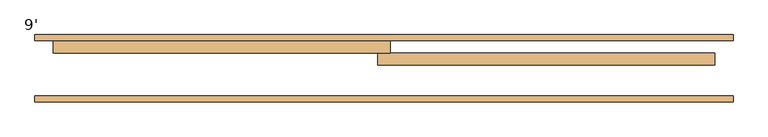
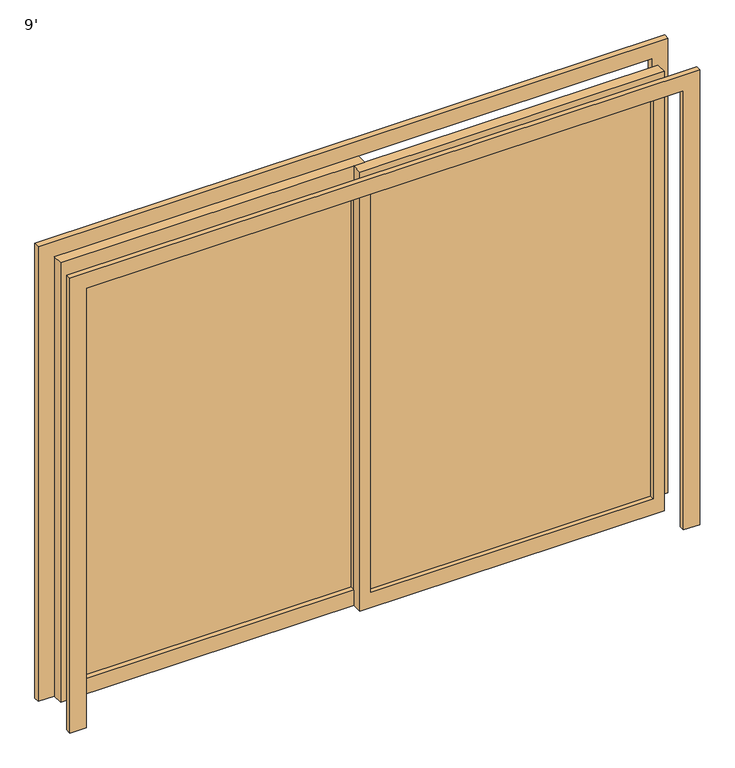
"""IFC4 building model written with IfcOpenShell, lengths in millimetres: door geometry, 9'."""

from ifc_helpers import new_model, si_unit, frame, origin, place, context, project, spatial, polyline, outline, extrude, source, transform, mapped, element, save


def door_9_db2a89ef(model_context):
    return source(origin(), model_context, "Body", "SweptSolid", [
        extrude(outline(polyline([(0.0, 1446.6), (2209.0, 1446.6), (2209.0, -1446.6), (0.0, -1446.6), (0.0, -1371.6), (2134.0, -1371.6), (2134.0, 1371.6), (0.0, 1371.6), (0.0, 1446.6)])), frame((0.0, 241.3, 0.0), z_axis=(0.0, 1.0, 0.0), x_axis=(0.0, 0.0, 1.0)), (0.0, 0.0, 1.0), 25.0),
        extrude(outline(polyline([(0.0, -1446.6), (0.0, -1371.6), (2134.0, -1371.6), (2134.0, 1371.6), (0.0, 1371.6), (0.0, 1446.6), (2209.0, 1446.6), (2209.0, -1446.6), (0.0, -1446.6)])), frame((0.0, -12.3, 0.0), z_axis=(0.0, 1.0, 0.0), x_axis=(0.0, 0.0, 1.0)), (0.0, 0.0, 1.0), 25.0),
        extrude(outline(polyline([(2134.0, 25.4), (2134.0, -1371.6), (0.0, -1371.6), (0.0, 25.4), (2134.0, 25.4)]), holes=[polyline([(2059.0, -24.6), (75.0, -24.6), (75.0, -1321.6), (2059.0, -1321.6), (2059.0, -24.6)])]), frame((0.0, 191.3, 0.0), z_axis=(0.0, 1.0, 0.0), x_axis=(0.0, 0.0, 1.0)), (0.0, 0.0, 1.0), 50.0),
        extrude(outline(polyline([(-1321.6, 219.475), (-24.6, 219.475), (-24.6, 213.125), (-1321.6, 213.125), (-1321.6, 219.475)])), frame((0.0, 0.0, 75.0), z_axis=(0.0, 0.0, 1.0), x_axis=(1.0, 0.0, 0.0)), (0.0, 0.0, 1.0), 1984.0),
        extrude(outline(polyline([(2134.0, -25.4), (0.0, -25.4), (0.0, 1371.6), (2134.0, 1371.6), (2134.0, -25.4)]), holes=[polyline([(2059.0, 24.6), (2059.0, 1321.6), (75.0, 1321.6), (75.0, 24.6), (2059.0, 24.6)])]), frame((0.0, 141.3, 0.0), z_axis=(0.0, 1.0, 0.0), x_axis=(0.0, 0.0, 1.0)), (0.0, 0.0, 1.0), 50.0),
        extrude(outline(polyline([(25.4, 169.475), (1321.6, 169.475), (1321.6, 163.125), (25.4, 163.125), (25.4, 169.475)])), frame((0.0, 0.0, 75.0), z_axis=(0.0, 0.0, 1.0), x_axis=(1.0, 0.0, 0.0)), (0.0, 0.0, 1.0), 1984.0),
    ])


if __name__ == "__main__":
    model = new_model("IFC4")
    model_context = context("Model", 3, world=origin())
    ifc_project = project(units=[si_unit("LENGTHUNIT", "METRE", prefix="MILLI")], contexts=[model_context])
    site = spatial("IfcSite", under=ifc_project)
    building = spatial("IfcBuilding", under=site)
    placement = place(None, origin())
    door_9_shape = door_9_db2a89ef(model_context)
    element("IfcDoor", 1, ObjectType="9'", at=placement, inside=building, context=model_context, shape_type="MappedRepresentation", body=[
        mapped(door_9_shape, transform((0.0, 0.0, 0.0), x_axis=(1.0, 0.0, 0.0), y_axis=(0.0, 1.0, 0.0), z_axis=(0.0, 0.0, 1.0))),
    ])
    save(model, "model.ifc")

# Revit data of these elements
# Type "9'"
#   Type Mark = "57"
#   Thickness = 0' - 1.9685"
#   Height = 7' - 0.01575"
#   Anchura de barandal = 0' - 2.95276"
#   Anchura de montante = 0' - 1.9685"
#   Proyección cubrejuntas ext. = 0' - 0.98425"
#   Proyección cubrejuntas int. = 0' - 0.98425"
#   Anchura de cubrejuntas = 0' - 2.95276"
#   Width = 9' - 0"
#   Material de puerta = Puerta - Panel
#   Function = (empty or 0)
#   Assembly Code = ""
#   Wall Closure = (empty or 0)
# Element 1 (IfcDoor, "9'")
#   Materials on its faces: "Puerta - Panel", "Cristal"
# Materials
#   "Puerta - Panel": class "Madera", colour RGB 210 159 95, transparency 0
#   "Cristal": class "Vidrio", colour RGB 0 0 255, transparency 0.75
